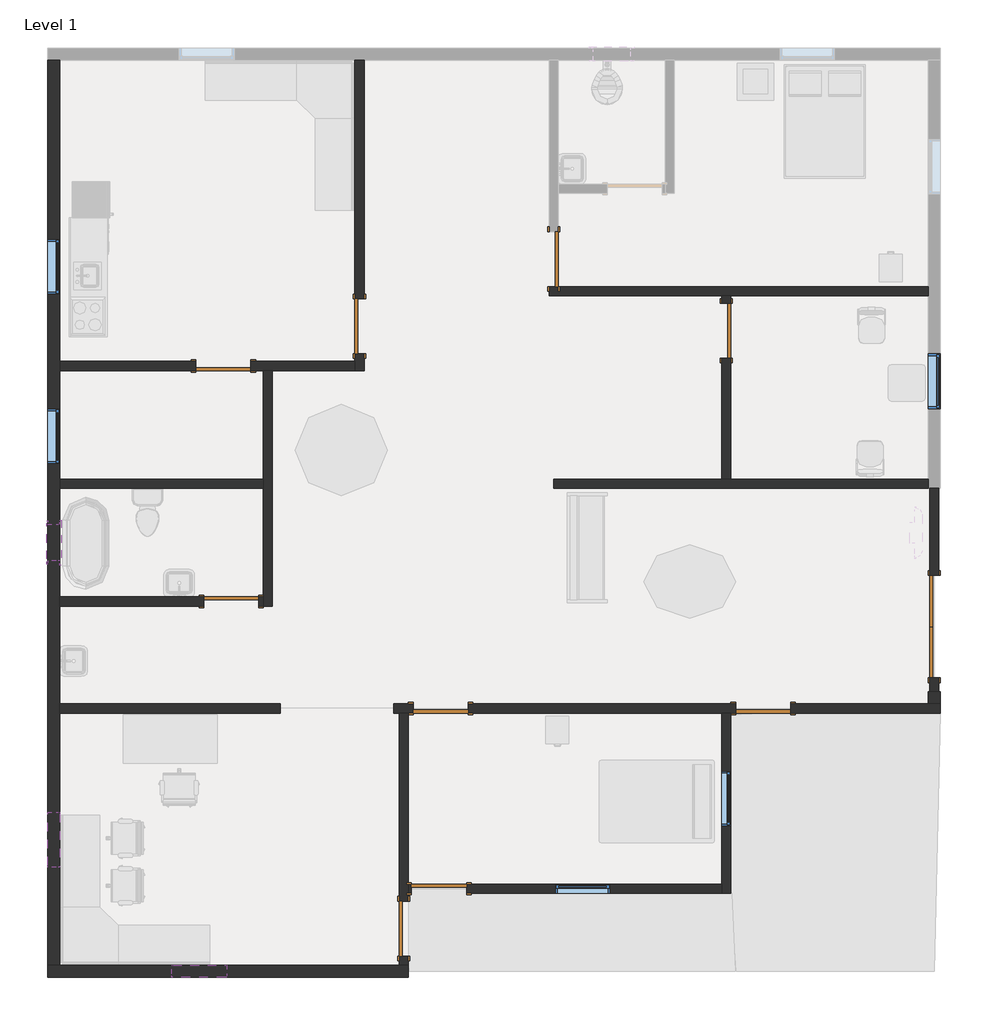
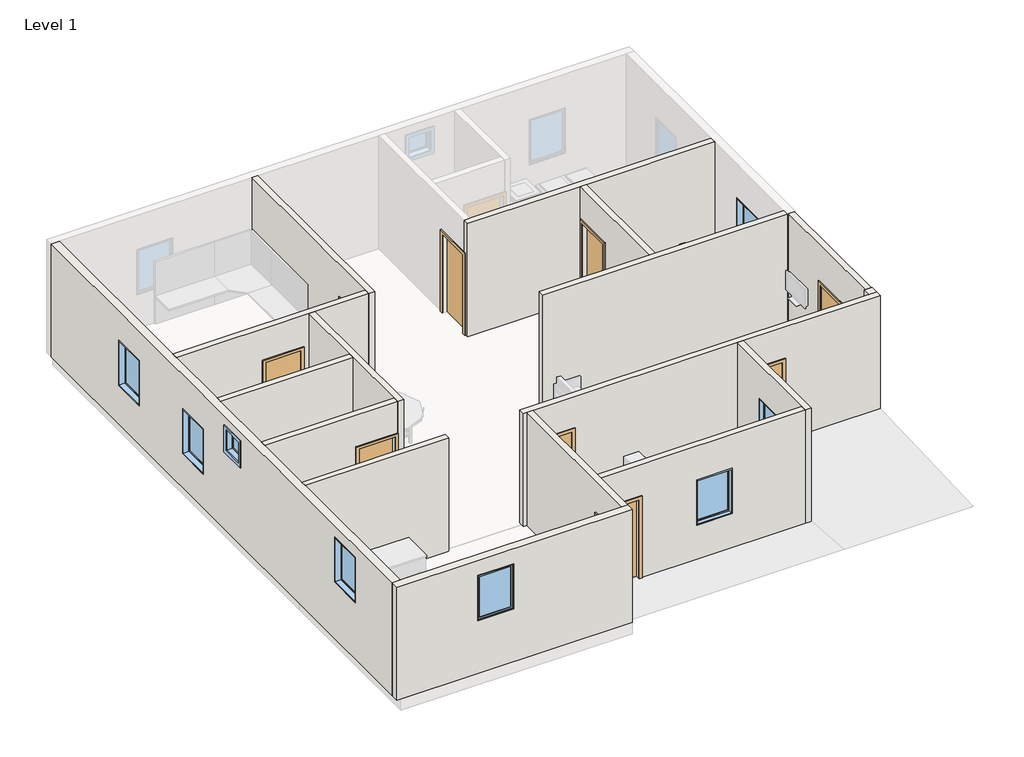
# One storey, part 1 of 2: 17 walls, 10 doors, 8 windows.
"""IFC4 building model written with IfcOpenShell, lengths in millimetres."""

from ifc_helpers import new_model, si_unit, frame, origin, origin_with_axes, place, context, project, spatial, polyline, outline, extrude, faceted_brep, transform, mapped, element, save
from components import m_door_double_flush_panel_1700_x_2000mm_b668bbd0, door_686f89d2, door_16372e1c, window_e2841890, window_d657a5cb, window_e41d21a6

model = new_model("IFC4")

# Units and contexts
model_context = context("Model", 3, world=origin())
ifc_project = project(units=[si_unit("LENGTHUNIT", "METRE", prefix="MILLI")], contexts=[model_context])

# Site, building, storey
site = spatial("IfcSite", under=ifc_project)
building = spatial("IfcBuilding", under=site)
storey = spatial("IfcBuildingStorey", under=building, Name="Level 1", Elevation=0.0)

# Doors
placement = place(None, origin())
m_door_double_flush_panel_1700_x_2000mm_shape = m_door_double_flush_panel_1700_x_2000mm_b668bbd0(model_context)
element("IfcDoor", 1, ObjectType="M_Door-Double-Flush_Panel : 1700 x 2000mm", at=placement, inside=storey, context=model_context, shape_type="MappedRepresentation", body=[
    mapped(m_door_double_flush_panel_1700_x_2000mm_shape, transform((-650.2737976, 1065.150395, 0.0), x_axis=(0.0, 1.0, 0.0), y_axis=(-1.0, 0.0, 0.0), z_axis=(0.0, 0.0, 1.0))),
])
door_shape = door_686f89d2(model_context)
element("IfcDoor", 2, ObjectType="Single-Flush : 36\" x 84\"", at=placement, inside=storey, context=model_context, shape_type="MappedRepresentation", body=[
    mapped(door_shape, transform((-10200.6737976, 6056.250395, 0.0), x_axis=(0.0, -1.0, 0.0), y_axis=(1.0, 0.0, 0.0), z_axis=(0.0, 0.0, 1.0))),
])
element("IfcDoor", 3, ObjectType="Single-Flush : 36\" x 84\"", at=placement, inside=storey, context=model_context, shape_type="MappedRepresentation", body=[
    mapped(door_shape, transform((-12461.2737976, 5395.850395, 0.0), x_axis=(1.0, 0.0, 0.0), y_axis=(0.0, 1.0, 0.0), z_axis=(0.0, 0.0, 1.0))),
])
element("IfcDoor", 4, ObjectType="Single-Flush : 36\" x 84\"", at=placement, inside=storey, context=model_context, shape_type="MappedRepresentation", body=[
    mapped(door_shape, transform((-9464.0737976, -3951.349605, 0.0), x_axis=(0.0, -1.0, 0.0), y_axis=(1.0, 0.0, 0.0), z_axis=(0.0, 0.0, 1.0))),
])
element("IfcDoor", 5, ObjectType="Single-Flush : 36\" x 84\"", at=placement, inside=storey, context=model_context, shape_type="MappedRepresentation", body=[
    mapped(door_shape, transform((-8879.8737976, -3290.949605, 0.0), x_axis=(-1.0, 0.0, 0.0), y_axis=(0.0, -1.0, 0.0), z_axis=(0.0, 0.0, 1.0))),
])
element("IfcDoor", 6, ObjectType="Single-Flush : 36\" x 84\"", at=placement, inside=storey, context=model_context, shape_type="MappedRepresentation", body=[
    mapped(door_shape, transform((-4104.6737976, 5980.050395, 0.0), x_axis=(0.0, 1.0, 0.0), y_axis=(-1.0, 0.0, 0.0), z_axis=(0.0, 0.0, 1.0))),
])
door_2_shape = door_16372e1c(model_context)
element("IfcDoor", 7, ObjectType="Single-Flush : 36\" x 84\"", at=placement, inside=storey, context=model_context, shape_type="MappedRepresentation", body=[
    mapped(door_2_shape, transform((-12334.2737976, 1484.250395, 0.0), x_axis=(1.0, 0.0, 0.0), y_axis=(0.0, 1.0, 0.0), z_axis=(0.0, 0.0, 1.0))),
])
element("IfcDoor", 8, ObjectType="Single-Flush : 36\" x 84\"", at=placement, inside=storey, context=model_context, shape_type="MappedRepresentation", body=[
    mapped(door_2_shape, transform((-8854.4737976, -293.749605, 0.0), x_axis=(-1.0, 0.0, 0.0), y_axis=(0.0, -1.0, 0.0), z_axis=(0.0, 0.0, 1.0))),
])
element("IfcDoor", 9, ObjectType="Single-Flush : 36\" x 84\"", at=placement, inside=storey, context=model_context, shape_type="MappedRepresentation", body=[
    mapped(door_2_shape, transform((-3495.0737976, -293.749605, 0.0), x_axis=(-1.0, 0.0, 0.0), y_axis=(0.0, -1.0, 0.0), z_axis=(0.0, 0.0, 1.0))),
])
element("IfcDoor", 10, ObjectType="Single-Flush : 36\" x 84\"", at=placement, inside=storey, context=model_context, shape_type="MappedRepresentation", body=[
    mapped(door_2_shape, transform((-6974.8737976, 7173.850395, 0.0), x_axis=(0.0, -1.0, 0.0), y_axis=(1.0, 0.0, 0.0), z_axis=(0.0, 0.0, 1.0))),
])

# Walls
element("IfcWall", 11, ObjectType="Generic - 8\"", at=placement, inside=storey, context=model_context, shape_type="Brep", body=[
    faceted_brep([(-15179.0737976, -4560.949605, 0.0), (-15179.0737976, -369.949605, 0.0), (-15179.0737976, -217.549605, 0.0), (-15179.0737976, 1408.050395, 0.0), (-15179.0737976, 1560.450395, 0.0), (-15179.0737976, 3363.850395, 0.0), (-15179.0737976, 3516.250395, 0.0), (-15179.0737976, 5319.650395, 0.0), (-15179.0737976, 5472.050395, 0.0), (-15179.0737976, 10475.850395, 0.0), (-15179.0737976, 10475.850395, 3048.0), (-15179.0737976, 5472.050395, 3048.0), (-15179.0737976, 5319.650395, 3048.0), (-15179.0737976, 3516.250395, 3048.0), (-15179.0737976, 3363.850395, 3048.0), (-15179.0737976, 1560.450395, 3048.0), (-15179.0737976, 1408.050395, 3048.0), (-15179.0737976, -217.549605, 3048.0), (-15179.0737976, -369.949605, 3048.0), (-15179.0737976, -4560.949605, 3048.0), (-15179.0737976, 6589.650395, 2260.6), (-15179.0737976, 7504.050395, 2260.6), (-15179.0737976, 7504.050395, 1041.4), (-15179.0737976, 6589.650395, 1041.4), (-15179.0737976, 3770.250395, 2133.6), (-15179.0737976, 4684.650395, 2133.6), (-15179.0737976, 4684.650395, 914.4), (-15179.0737976, 3770.250395, 914.4), (-15179.0737976, -2935.349605, 2743.2), (-15179.0737976, -2020.949605, 2743.2), (-15179.0737976, -2020.949605, 1524.0), (-15179.0737976, -2935.349605, 1524.0), (-15179.0737976, 2157.350395, 2768.6), (-15179.0737976, 2766.950395, 2768.6), (-15179.0737976, 2766.950395, 2159.0), (-15179.0737976, 2157.350395, 2159.0), (-15382.2737976, -4560.949605, 0.0), (-15382.2737976, -4560.949605, 3048.0), (-15382.2737976, 10475.850395, 3048.0), (-15382.2737976, 10475.850395, 0.0), (-15382.2737976, 6589.650395, 2260.6), (-15382.2737976, 6589.650395, 1041.4), (-15382.2737976, 7504.050395, 1041.4), (-15382.2737976, 7504.050395, 2260.6), (-15382.2737976, 3770.250395, 2133.6), (-15382.2737976, 3770.250395, 914.4), (-15382.2737976, 4684.650395, 914.4), (-15382.2737976, 4684.650395, 2133.6), (-15382.2737976, -2935.349605, 2743.2), (-15382.2737976, -2935.349605, 1524.0), (-15382.2737976, -2020.949605, 1524.0), (-15382.2737976, -2020.949605, 2743.2), (-15382.2737976, 2157.350395, 2768.6), (-15382.2737976, 2157.350395, 2159.0), (-15382.2737976, 2766.950395, 2159.0), (-15382.2737976, 2766.950395, 2768.6)], [[[0, 1, 2, 3, 4, 5, 6, 7, 8, 9, 10, 11, 12, 13, 14, 15, 16, 17, 18, 19], [20, 21, 22, 23], [24, 25, 26, 27], [28, 29, 30, 31], [32, 33, 34, 35]], [[36, 37, 38, 39], [40, 41, 42, 43], [44, 45, 46, 47], [48, 49, 50, 51], [52, 53, 54, 55]], [[9, 8, 7, 6, 5, 4, 3, 2, 1, 0, 36, 39]], [[19, 18, 17, 16, 15, 14, 13, 12, 11, 10, 38, 37]], [[10, 9, 39, 38]], [[0, 19, 37, 36]], [[41, 40, 20, 23]], [[42, 41, 23, 22]], [[43, 42, 22, 21]], [[40, 43, 21, 20]], [[45, 44, 24, 27]], [[46, 45, 27, 26]], [[47, 46, 26, 25]], [[44, 47, 25, 24]], [[49, 48, 28, 31]], [[50, 49, 31, 30]], [[51, 50, 30, 29]], [[48, 51, 29, 28]], [[53, 52, 32, 35]], [[54, 53, 35, 34]], [[55, 54, 34, 33]], [[52, 55, 33, 32]]]),
])
element("IfcWall", 12, ObjectType="Generic - 8\"", at=placement, inside=storey, context=model_context, shape_type="Brep", body=[
    faceted_brep([(-9387.8737976, -4560.949605, 0.0), (-9540.2737976, -4560.949605, 0.0), (-15179.0737976, -4560.949605, 0.0), (-15382.2737976, -4560.949605, 0.0), (-15382.2737976, -4560.949605, 3048.0), (-15179.0737976, -4560.949605, 3048.0), (-9540.2737976, -4560.949605, 3048.0), (-9387.8737976, -4560.949605, 3048.0), (-13324.8737976, -4560.949605, 2641.6), (-13324.8737976, -4560.949605, 1422.4), (-12410.4737976, -4560.949605, 1422.4), (-12410.4737976, -4560.949605, 2641.6), (-9387.8737976, -4764.149605, 0.0), (-9387.8737976, -4764.149605, 3048.0), (-15382.2737976, -4764.149605, 3048.0), (-15382.2737976, -4764.149605, 0.0), (-13324.8737976, -4764.149605, 2641.6), (-12410.4737976, -4764.149605, 2641.6), (-12410.4737976, -4764.149605, 1422.4), (-13324.8737976, -4764.149605, 1422.4)], [[[0, 1, 2, 3, 4, 5, 6, 7], [8, 9, 10, 11]], [[12, 13, 14, 15], [16, 17, 18, 19]], [[3, 2, 1, 0, 12, 15]], [[7, 6, 5, 4, 14, 13]], [[4, 3, 15, 14]], [[0, 7, 13, 12]], [[9, 8, 16, 19]], [[10, 9, 19, 18]], [[11, 10, 18, 17]], [[8, 11, 17, 16]]]),
])
element("IfcWall", 13, ObjectType="Generic - 8\"", at=placement, inside=storey, context=model_context, shape_type="Brep", body=[
    faceted_brep([(-751.8737976, -14.349605, 0.0), (-751.8737976, -217.549605, 0.0), (-751.8737976, -217.549605, 3048.0), (-751.8737976, -14.349605, 3048.0), (-548.6737976, -14.349605, 0.0), (-548.6737976, -14.349605, 3048.0), (-548.6737976, -217.549605, 3048.0), (-548.6737976, -217.549605, 0.0), (-726.4737976, -14.349605, 0.0), (-574.0737976, -14.349605, 0.0), (-574.0737976, -14.349605, 3048.0), (-726.4737976, -14.349605, 3048.0)], [[[0, 1, 2, 3]], [[4, 5, 6, 7]], [[1, 0, 8, 9, 4, 7]], [[3, 2, 6, 5, 10, 11]], [[0, 3, 11, 10, 5, 4, 9, 8]], [[2, 1, 7, 6]]]),
])
element("IfcWall", 14, ObjectType="INNER WALL 6\"", at=placement, inside=storey, context=model_context, shape_type="Brep", body=[
    faceted_brep([(-10276.8737976, 5599.050395, 2133.6), (-10276.8737976, 5599.050395, 0.0), (-10276.8737976, 5472.050395, 0.0), (-10276.8737976, 5319.650395, 0.0), (-10276.8737976, 5319.650395, 3048.0), (-10276.8737976, 5472.050395, 3048.0), (-10276.8737976, 10475.850395, 3048.0), (-10276.8737976, 10475.850395, 0.0), (-10276.8737976, 6513.450395, 0.0), (-10276.8737976, 6513.450395, 2133.6), (-10124.4737976, 5319.650395, 0.0), (-10124.4737976, 5599.050395, 0.0), (-10124.4737976, 5599.050395, 2133.6), (-10124.4737976, 6513.450395, 2133.6), (-10124.4737976, 6513.450395, 0.0), (-10124.4737976, 10475.850395, 0.0), (-10124.4737976, 10475.850395, 3048.0), (-10124.4737976, 5319.650395, 3048.0)], [[[0, 1, 2, 3, 4, 5, 6, 7, 8, 9]], [[10, 11, 12, 13, 14, 15, 16, 17]], [[8, 7, 15, 14]], [[3, 2, 1, 11, 10]], [[6, 5, 4, 17, 16]], [[7, 6, 16, 15]], [[4, 3, 10, 17]], [[12, 11, 1, 0]], [[13, 12, 0, 9]], [[14, 13, 9, 8]]]),
])
element("IfcWall", 15, ObjectType="INNER WALL 6\"", at=placement, inside=storey, context=model_context, shape_type="Brep", body=[
    faceted_brep([(-10276.8737976, 5472.050395, 0.0), (-12004.0737976, 5472.050395, 0.0), (-12004.0737976, 5472.050395, 2133.6), (-12918.4737976, 5472.050395, 2133.6), (-12918.4737976, 5472.050395, 0.0), (-15179.0737976, 5472.050395, 0.0), (-15179.0737976, 5472.050395, 3048.0), (-10276.8737976, 5472.050395, 3048.0), (-12004.0737976, 5319.650395, 2133.6), (-12004.0737976, 5319.650395, 0.0), (-11800.8737976, 5319.650395, 0.0), (-11648.4737976, 5319.650395, 0.0), (-10276.8737976, 5319.650395, 0.0), (-10276.8737976, 5319.650395, 3048.0), (-11648.4737976, 5319.650395, 3048.0), (-11800.8737976, 5319.650395, 3048.0), (-15179.0737976, 5319.650395, 3048.0), (-15179.0737976, 5319.650395, 0.0), (-12918.4737976, 5319.650395, 0.0), (-12918.4737976, 5319.650395, 2133.6)], [[[0, 1, 2, 3, 4, 5, 6, 7]], [[8, 9, 10, 11, 12, 13, 14, 15, 16, 17, 18, 19]], [[18, 17, 5, 4]], [[12, 11, 10, 9, 1, 0]], [[7, 6, 16, 15, 14, 13]], [[0, 7, 13, 12]], [[6, 5, 17, 16]], [[2, 1, 9, 8]], [[3, 2, 8, 19]], [[4, 3, 19, 18]]]),
])
element("IfcWall", 16, ObjectType="INNER WALL 6\"", at=placement, inside=storey, context=model_context, shape_type="Brep", body=[
    faceted_brep([(-11800.8737976, 5319.650395, 0.0), (-11800.8737976, 3516.250395, 0.0), (-11800.8737976, 3363.850395, 0.0), (-11800.8737976, 1560.450395, 0.0), (-11800.8737976, 1408.050395, 0.0), (-11800.8737976, 1408.050395, 3048.0), (-11800.8737976, 1560.450395, 3048.0), (-11800.8737976, 3363.850395, 3048.0), (-11800.8737976, 3516.250395, 3048.0), (-11800.8737976, 5319.650395, 3048.0), (-11648.4737976, 5319.650395, 0.0), (-11648.4737976, 5319.650395, 3048.0), (-11648.4737976, 1408.050395, 3048.0), (-11648.4737976, 1408.050395, 0.0)], [[[0, 1, 2, 3, 4, 5, 6, 7, 8, 9]], [[10, 11, 12, 13]], [[4, 3, 2, 1, 0, 10, 13]], [[9, 8, 7, 6, 5, 12, 11]], [[0, 9, 11, 10]], [[5, 4, 13, 12]]]),
])
element("IfcWall", 17, ObjectType="INNER WALL 6\"", at=placement, inside=storey, context=model_context, shape_type="SweptSolid", body=[
    extrude(outline(polyline([(2133.6, -11877.0737976), (0.0, -11877.0737976), (0.0, -11800.8737976), (3048.0, -11800.8737976), (3048.0, -15179.0737976), (0.0, -15179.0737976), (0.0, -12791.4737976), (2133.6, -12791.4737976), (2133.6, -11877.0737976)])), frame((0.0, 1408.050395, 0.0), z_axis=(0.0, 1.0, 0.0), x_axis=(0.0, 0.0, 1.0)), (0.0, 0.0, 1.0), 152.4),
])
element("IfcWall", 18, ObjectType="INNER WALL 6\"", at=placement, inside=storey, context=model_context, shape_type="SweptSolid", body=[
    extrude(outline(polyline([(-15179.0737976, 3516.250395), (-11800.8737976, 3516.250395), (-11800.8737976, 3363.850395), (-15179.0737976, 3363.850395), (-15179.0737976, 3516.250395)])), origin_with_axes(), (0.0, 0.0, 1.0), 3048.0),
])
element("IfcWall", 19, ObjectType="INNER WALL 6\"", at=placement, inside=storey, context=model_context, shape_type="SweptSolid", body=[
    extrude(outline(polyline([(-11521.4737976, -369.949605), (-15179.0737976, -369.949605), (-15179.0737976, -217.549605), (-11521.4737976, -217.549605), (-11521.4737976, -369.949605)])), origin_with_axes(), (0.0, 0.0, 1.0), 3048.0),
])
element("IfcWall", 20, ObjectType="INNER WALL 6\"", at=placement, inside=storey, context=model_context, shape_type="Brep", body=[
    faceted_brep([(-9540.2737976, -4408.549605, 2133.6), (-9540.2737976, -4408.549605, 0.0), (-9540.2737976, -4560.949605, 0.0), (-9540.2737976, -4560.949605, 3048.0), (-9540.2737976, -369.949605, 3048.0), (-9540.2737976, -369.949605, 0.0), (-9540.2737976, -3494.149605, 0.0), (-9540.2737976, -3494.149605, 2133.6), (-9387.8737976, -4560.949605, 0.0), (-9387.8737976, -4408.549605, 0.0), (-9387.8737976, -4408.549605, 2133.6), (-9387.8737976, -3494.149605, 2133.6), (-9387.8737976, -3494.149605, 0.0), (-9387.8737976, -3367.149605, 0.0), (-9387.8737976, -3214.749605, 0.0), (-9387.8737976, -369.949605, 0.0), (-9387.8737976, -369.949605, 3048.0), (-9387.8737976, -3214.749605, 3048.0), (-9387.8737976, -3367.149605, 3048.0), (-9387.8737976, -4560.949605, 3048.0)], [[[0, 1, 2, 3, 4, 5, 6, 7]], [[8, 9, 10, 11, 12, 13, 14, 15, 16, 17, 18, 19]], [[6, 5, 15, 14, 13, 12]], [[2, 1, 9, 8]], [[4, 3, 19, 18, 17, 16]], [[5, 4, 16, 15]], [[10, 9, 1, 0]], [[11, 10, 0, 7]], [[12, 11, 7, 6]], [[3, 2, 8, 19]]]),
])
element("IfcWall", 21, ObjectType="INNER WALL 6\"", at=placement, inside=storey, context=model_context, shape_type="Brep", body=[
    faceted_brep([(-4180.8737976, -369.949605, 0.0), (-4180.8737976, -3214.749605, 0.0), (-4180.8737976, -3367.149605, 0.0), (-4180.8737976, -3367.149605, 3048.0), (-4180.8737976, -3214.749605, 3048.0), (-4180.8737976, -369.949605, 3048.0), (-4180.8737976, -2249.549605, 2133.6), (-4180.8737976, -2249.549605, 914.4), (-4180.8737976, -1335.149605, 914.4), (-4180.8737976, -1335.149605, 2133.6), (-4028.4737976, -369.949605, 0.0), (-4028.4737976, -369.949605, 3048.0), (-4028.4737976, -3367.149605, 3048.0), (-4028.4737976, -3367.149605, 0.0), (-4028.4737976, -2249.549605, 2133.6), (-4028.4737976, -1335.149605, 2133.6), (-4028.4737976, -1335.149605, 914.4), (-4028.4737976, -2249.549605, 914.4)], [[[0, 1, 2, 3, 4, 5], [6, 7, 8, 9]], [[10, 11, 12, 13], [14, 15, 16, 17]], [[2, 1, 0, 10, 13]], [[5, 4, 3, 12, 11]], [[3, 2, 13, 12]], [[0, 5, 11, 10]], [[7, 6, 14, 17]], [[8, 7, 17, 16]], [[9, 8, 16, 15]], [[6, 9, 15, 14]]]),
])
element("IfcWall", 22, ObjectType="INNER WALL 6\"", at=placement, inside=storey, context=model_context, shape_type="Brep", body=[
    faceted_brep([(-6974.8737976, 3363.850395, 0.0), (-751.8737976, 3363.850395, 0.0), (-751.8737976, 3363.850395, 3048.0), (-6974.8737976, 3363.850395, 3048.0), (-6974.8737976, 3516.250395, 0.0), (-6974.8737976, 3516.250395, 3048.0), (-4180.8737976, 3516.250395, 3048.0), (-4028.4737976, 3516.250395, 3048.0), (-751.8737976, 3516.250395, 3048.0), (-751.8737976, 3516.250395, 0.0), (-4028.4737976, 3516.250395, 0.0), (-4180.8737976, 3516.250395, 0.0)], [[[0, 1, 2, 3]], [[4, 5, 6, 7, 8, 9, 10, 11]], [[1, 0, 4, 11, 10, 9]], [[3, 2, 8, 7, 6, 5]], [[0, 3, 5, 4]], [[2, 1, 9, 8]]]),
])
element("IfcWall", 23, ObjectType="INNER WALL 6\"", at=placement, inside=storey, context=model_context, shape_type="SweptSolid", body=[
    extrude(outline(polyline([(6564.250395, 0.0), (6437.250395, 0.0), (6437.250395, 2133.6), (5522.850395, 2133.6), (5522.850395, 0.0), (3516.250395, 0.0), (3516.250395, 3048.0), (6564.250395, 3048.0), (6564.250395, 0.0)])), frame((-4180.8737976, 0.0, 0.0), z_axis=(1.0, 0.0, 0.0), x_axis=(0.0, 1.0, 0.0)), (0.0, 0.0, 1.0), 152.4),
])
element("IfcWall", 24, ObjectType="INNER WALL 6\"", at=placement, inside=storey, context=model_context, shape_type="Brep", body=[
    faceted_brep([(-7051.0737976, 6564.250395, 0.0), (-4180.8737976, 6564.250395, 0.0), (-4028.4737976, 6564.250395, 0.0), (-751.8737976, 6564.250395, 0.0), (-751.8737976, 6564.250395, 3048.0), (-4028.4737976, 6564.250395, 3048.0), (-4180.8737976, 6564.250395, 3048.0), (-7051.0737976, 6564.250395, 3048.0), (-7051.0737976, 6716.650395, 0.0), (-7051.0737976, 6716.650395, 2133.6), (-7051.0737976, 6716.650395, 3048.0), (-6898.6737976, 6716.650395, 3048.0), (-751.8737976, 6716.650395, 3048.0), (-751.8737976, 6716.650395, 0.0)], [[[0, 1, 2, 3, 4, 5, 6, 7]], [[8, 9, 10, 11, 12, 13]], [[3, 2, 1, 0, 8, 13]], [[7, 6, 5, 4, 12, 11, 10]], [[4, 3, 13, 12]], [[0, 7, 10, 9, 8]]]),
])
element("IfcWall", 25, ObjectType="INNER WALL 6\"", at=placement, inside=storey, context=model_context, shape_type="SweptSolid", body=[
    extrude(outline(polyline([(0.0, -9387.8737976), (0.0, -9337.0737976), (2133.6, -9337.0737976), (2133.6, -8422.6737976), (0.0, -8422.6737976), (0.0, -4180.8737976), (3048.0, -4180.8737976), (3048.0, -9387.8737976), (0.0, -9387.8737976)]), holes=[polyline([(2133.6, -6035.0737976), (914.4, -6035.0737976), (914.4, -6949.4737976), (2133.6, -6949.4737976), (2133.6, -6035.0737976)])]), frame((0.0, -3367.149605, 0.0), z_axis=(0.0, 1.0, 0.0), x_axis=(0.0, 0.0, 1.0)), (0.0, 0.0, 1.0), 152.4),
])
element("IfcWall", 26, ObjectType="INNER WALL 6\"", at=placement, inside=storey, context=model_context, shape_type="Brep", body=[
    faceted_brep([(-8397.2737976, -369.949605, 0.0), (-4180.8737976, -369.949605, 0.0), (-4028.4737976, -369.949605, 0.0), (-3952.2737976, -369.949605, 0.0), (-3952.2737976, -369.949605, 2133.6), (-3037.8737976, -369.949605, 2133.6), (-3037.8737976, -369.949605, 0.0), (-548.6737976, -369.949605, 0.0), (-548.6737976, -369.949605, 3048.0), (-4028.4737976, -369.949605, 3048.0), (-4180.8737976, -369.949605, 3048.0), (-9387.8737976, -369.949605, 3048.0), (-9540.2737976, -369.949605, 3048.0), (-9629.1737976, -369.949605, 3048.0), (-9629.1737976, -369.949605, 0.0), (-9540.2737976, -369.949605, 0.0), (-9387.8737976, -369.949605, 0.0), (-9311.6737976, -369.949605, 0.0), (-9311.6737976, -369.949605, 2133.6), (-8397.2737976, -369.949605, 2133.6), (-3952.2737976, -217.549605, 2133.6), (-3952.2737976, -217.549605, 0.0), (-8397.2737976, -217.549605, 0.0), (-8397.2737976, -217.549605, 2133.6), (-9311.6737976, -217.549605, 2133.6), (-9311.6737976, -217.549605, 0.0), (-9629.1737976, -217.549605, 0.0), (-9629.1737976, -217.549605, 3048.0), (-751.8737976, -217.549605, 3048.0), (-548.6737976, -217.549605, 3048.0), (-548.6737976, -217.549605, 0.0), (-751.8737976, -217.549605, 0.0), (-3037.8737976, -217.549605, 0.0), (-3037.8737976, -217.549605, 2133.6)], [[[0, 1, 2, 3, 4, 5, 6, 7, 8, 9, 10, 11, 12, 13, 14, 15, 16, 17, 18, 19]], [[20, 21, 22, 23, 24, 25, 26, 27, 28, 29, 30, 31, 32, 33]], [[26, 25, 17, 16, 15, 14]], [[22, 21, 3, 2, 1, 0]], [[32, 31, 30, 7, 6]], [[13, 12, 11, 10, 9, 8, 29, 28, 27]], [[14, 13, 27, 26]], [[8, 7, 30, 29]], [[0, 19, 23, 22]], [[19, 18, 24, 23]], [[18, 17, 25, 24]], [[6, 5, 33, 32]], [[5, 4, 20, 33]], [[4, 3, 21, 20]]]),
])
element("IfcWall", 27, ObjectType="INNER WALL 6\"", at=placement, inside=storey, context=model_context, shape_type="SweptSolid", body=[
    extrude(outline(polyline([(-14.349605, 3048.0), (3363.850395, 3048.0), (3363.850395, 0.0), (1915.150395, 0.0), (1915.150395, 2000.0), (215.150395, 2000.0), (215.150395, 0.0), (-14.349605, 0.0), (-14.349605, 3048.0)])), frame((-726.4737976, 0.0, 0.0), z_axis=(1.0, 0.0, 0.0), x_axis=(0.0, 1.0, 0.0)), (0.0, 0.0, 1.0), 152.4),
])

# Windows
window_shape = window_e2841890(model_context)
element("IfcWindow", 28, ObjectType="Fixed : 36\" x 48\"", at=placement, inside=storey, context=model_context, shape_type="MappedRepresentation", body=[
    mapped(window_shape, transform((-15280.6737976, 7008.750395, 127.0), x_axis=(0.0, -1.0, 0.0), y_axis=(1.0, 0.0, 0.0), z_axis=(0.0, 0.0, 1.0))),
])
element("IfcWindow", 29, ObjectType="Fixed : 36\" x 48\"", at=placement, inside=storey, context=model_context, shape_type="MappedRepresentation", body=[
    mapped(window_shape, transform((-15280.6737976, 4189.350395, 0.0), x_axis=(0.0, -1.0, 0.0), y_axis=(1.0, 0.0, 0.0), z_axis=(0.0, 0.0, 1.0))),
])
element("IfcWindow", 30, ObjectType="Fixed : 36\" x 48\"", at=placement, inside=storey, context=model_context, shape_type="MappedRepresentation", body=[
    mapped(window_shape, transform((-15280.6737976, -2516.249605, 609.6), x_axis=(0.0, -1.0, 0.0), y_axis=(1.0, 0.0, 0.0), z_axis=(0.0, 0.0, 1.0))),
])
element("IfcWindow", 31, ObjectType="Fixed : 36\" x 48\"", at=placement, inside=storey, context=model_context, shape_type="MappedRepresentation", body=[
    mapped(window_shape, transform((-12905.7737976, -4662.549605, 508.0), x_axis=(-1.0, 0.0, 0.0), y_axis=(0.0, -1.0, 0.0), z_axis=(0.0, 0.0, 1.0))),
])
element("IfcWindow", 32, ObjectType="Fixed : 36\" x 48\"", at=placement, inside=storey, context=model_context, shape_type="MappedRepresentation", body=[
    mapped(window_shape, transform((-650.2737976, 5103.750395, 0.0), x_axis=(0.0, -1.0, 0.0), y_axis=(1.0, 0.0, 0.0), z_axis=(0.0, 0.0, 1.0))),
])
window_2_shape = window_d657a5cb(model_context)
element("IfcWindow", 33, ObjectType="Fixed : 36\" x 48\"", at=placement, inside=storey, context=model_context, shape_type="MappedRepresentation", body=[
    mapped(window_2_shape, transform((-6454.1737976, -3290.949605, 0.0), x_axis=(1.0, 0.0, 0.0), y_axis=(0.0, 1.0, 0.0), z_axis=(0.0, 0.0, 1.0))),
])
element("IfcWindow", 34, ObjectType="Fixed : 36\" x 48\"", at=placement, inside=storey, context=model_context, shape_type="MappedRepresentation", body=[
    mapped(window_2_shape, transform((-4104.6737976, -1830.449605, 0.0), x_axis=(0.0, -1.0, 0.0), y_axis=(1.0, 0.0, 0.0), z_axis=(0.0, 0.0, 1.0))),
])
window_3_shape = window_e41d21a6(model_context)
element("IfcWindow", 35, ObjectType="Transom with Trim : 24\" x 24\"", at=placement, inside=storey, context=model_context, shape_type="MappedRepresentation", body=[
    mapped(window_3_shape, transform((-15280.6737976, 2424.050395, 0.0), x_axis=(0.0, -1.0, 0.0), y_axis=(1.0, 0.0, 0.0), z_axis=(0.0, 0.0, 1.0))),
])

save(model, "model.ifc")

# Revit data of these elements
# Type "M_Door-Double-Flush_Panel : 1700 x 2000mm"
#   Type Mark = "8"
#   Construction Type Id = "DOOR"
#   Assembly Code = "C1020"
#   Analytic Construction = "Wooden"
#   Thickness = 0' - 1.9685"
#   Thermal Resistance (R) = 2.5876 (h·ft²·°F)/BTU
#   Swing Angle [instance default] = 90.00°
#   Panel Width = 2' - 9.46457"
#   Heat Transfer Coefficient (U) = 0.3865 BTU/(h·ft²·°F)
#   Height = 6' - 6.74016"
#   Trim Projection Ext = 0' - 0.98425"
#   Trim Projection Int = 0' - 0.98425"
#   Trim Width = 0' - 3.14961"
#   Width = 5' - 6.92913"
#   Define Thermal Properties by = 1
#   Panel Material = Wood - Birch - Solid Stained Light Low Gloss
#   Trim Material = Paint - Sienna
#   Visual Light Transmittance = 0
#   Solar Heat Gain Coefficient = 0
#   Function = (empty or 0)
#   Wall Closure = (empty or 0)
# Type "Single-Flush : 36\" x 84\""
#   Type Mark = "1"
#   Construction Type Id = "MDOOR"
#   Assembly Code = "C1020"
#   Analytic Construction = "Metal"
#   Thickness = 0' - 2"
#   Heat Transfer Coefficient (U) = 0.651978 BTU/(h·ft²·°F)
#   Height = 7' - 0"
#   Trim Projection Ext = 0' - 1"
#   Trim Projection Int = 0' - 1"
#   Trim Width = 0' - 3"
#   Width = 3' - 0"
#   Define Thermal Properties by = 1
#   Door Material = Door - Panel
#   Frame Material = Door - Frame
#   Visual Light Transmittance = 0
#   Solar Heat Gain Coefficient = 0
#   Function = (empty or 0)
#   Wall Closure = (empty or 0)
# Type "Generic - 8\""
#   Assembly Code = "B2010"
#   Layers, outside or top first: 0' - 8" no material (function 1)
# Type "INNER WALL 6\""
#   Assembly Code = "B2010"
#   Layers, outside or top first: 0' - 6" no material (function 1)
# Type "Fixed : 36\" x 48\""
#   Type Mark = "1"
#   Construction Type Id = "GSP4R"
#   Assembly Code = "B2020100"
#   Analytic Construction = "1/8 in Pilkington single glazing"
#   Visual Light Transmittance = 0.9
#   Solar Heat Gain Coefficient = 0.78
#   Heat Transfer Coefficient (U) = 0.6496 BTU/(h·ft²·°F)
#   Height = 4' - 0"
#   Default Sill Height = 3' - 0"
#   Width = 3' - 0"
#   Window Inset = 0' - 0 3/4"
#   Define Thermal Properties by = 1
#   Glass Pane Material = Glass
#   Sash Material = Sash
#   Wall Closure = (empty or 0)
# Type "Transom with Trim : 24\" x 24\""
#   Type Mark = "10"
#   Construction Type Id = "GSP4R"
#   Assembly Code = "B2020100"
#   Analytic Construction = "1/8 in Pilkington single glazing"
#   Visual Light Transmittance = 0.9
#   Solar Heat Gain Coefficient = 0.78
#   Heat Transfer Coefficient (U) = 0.6496 BTU/(h·ft²·°F)
#   Height = 2' - 0"
#   Default Sill Height = 7' - 1"
#   Trim Projection - Ext. = 0' - 0 1/2"
#   Trim Projection - Int. = 0' - 0 3/4"
#   Trim Width - Exterior = 0' - 3 1/2"
#   Trim Width - Interior = 0' - 3 1/2"
#   Width = 2' - 0"
#   Window Inset = 0' - 0 3/4"
#   Define Thermal Properties by = 1
#   Glass Pane Material = Glass
#   Sash Material = Sash
#   Trim Exterior Material = Trim
#   Trim Interior Material = Trim
#   Wall Closure = (empty or 0)
# Element 1 (IfcDoor, "M_Door-Double-Flush_Panel : 1700 x 2000mm")
#   Swing Angle = 90.00°
#   Phase Created = New Construction
#   Materials on its faces: "Paint - Sienna", "Wood - Birch - Solid Stained Light Low Gloss"
# Elements 2, 3, 4, 5, 6, 7, 8, 9, 10 (IfcDoor, "Single-Flush : 36\" x 84\"")
#   Phase Created = New Construction
#   Materials on its faces: "Door - Frame", "Door - Panel"
# Elements 11, 12, 13 (IfcWall, "Generic - 8\"")
#   Top Offset = 0' - 0"
#   Base Offset = 0' - 0"
#   Unconnected Height = 10' - 0"
#   wall height = 10' - 0"
#   Phase Created = New Construction
#   Base Constraint = Level 1
#   Materials on its faces: "Default Wall"
# Elements 14, 15, 16, 17, 18, 19, 20, 21, 22, 23, 24, 25, 26, 27 (IfcWall, "INNER WALL 6\"")
#   Top Offset = 0' - 0"
#   Base Offset = 0' - 0"
#   Unconnected Height = 10' - 0"
#   wall height = 10' - 0"
#   Phase Created = New Construction
#   Base Constraint = Level 1
#   Materials on its faces: "Default Wall"
# Element 28 (IfcWindow, "Fixed : 36\" x 48\"")
#   Mark = "2"
#   Phase Created = New Construction
#   Materials on its faces: "Sash", "Glass"
# Element 29 (IfcWindow, "Fixed : 36\" x 48\"")
#   Mark = "3"
#   Phase Created = New Construction
#   Materials on its faces: "Sash", "Glass"
# Element 30 (IfcWindow, "Fixed : 36\" x 48\"")
#   Mark = "5"
#   Phase Created = New Construction
#   Materials on its faces: "Sash", "Glass"
# Element 31 (IfcWindow, "Fixed : 36\" x 48\"")
#   Mark = "6"
#   Phase Created = New Construction
#   Materials on its faces: "Sash", "Glass"
# Element 32 (IfcWindow, "Fixed : 36\" x 48\"")
#   Mark = "10"
#   Phase Created = New Construction
#   Materials on its faces: "Sash", "Glass"
# Element 33 (IfcWindow, "Fixed : 36\" x 48\"")
#   Mark = "7"
#   Phase Created = New Construction
#   Materials on its faces: "Sash", "Glass"
# Element 34 (IfcWindow, "Fixed : 36\" x 48\"")
#   Mark = "8"
#   Phase Created = New Construction
#   Materials on its faces: "Sash", "Glass"
# Element 35 (IfcWindow, "Transom with Trim : 24\" x 24\"")
#   Mark = "13"
#   Phase Created = New Construction
#   Materials on its faces: "Sash", "Trim", "Glass"
# Materials
#   "Wood - Birch - Solid Stained Light Low Gloss": class "Wood", colour RGB 210 159 95, transparency 0, Cost = 0
#   "Paint - Sienna": colour RGB 118 70 51, transparency 0, Cost = 0
#   "Door - Panel": class "Wood", colour RGB 210 159 95, transparency 0
#   "Door - Frame": colour RGB 118 70 51, transparency 0
#   "Glass": class "Glass", colour RGB 0 128 192, transparency 0.75, Description = "Soda Lime Glass", Cost = 0
#   "Sash": class "Wood", colour RGB 224 178 126, transparency 0
#   "Trim": class "Wood", colour RGB 224 178 126, transparency 0
#   "Default Wall": colour RGB 128 128 128, transparency 0
# Room at (-8814.416, 8901.561) mm, phase "New Construction", upper level "Level 1", upper offset 10' - 0", lower offset 0' - 0"
#   Number = "10"
#   Name = "WASH AREA"
# Room at (-5691.492, 9434.245) mm, phase "New Construction", upper level "Level 1", upper offset 10' - 0", lower offset 0' - 0"
#   Number = "11"
# Room at (-2665.543, 8172.09) mm, phase "New Construction", upper level "Level 1", upper offset 10' - 0", lower offset 0' - 0"
#   Number = "12"
#   Name = "BED ROOM"
# Room at (-13037.673, 7334.606) mm, phase "New Construction", upper level "Level 1", upper offset 10' - 0", lower offset 0' - 0"
#   Number = "1"
#   Name = "KITCHEN ROOM"
# Room at (-13302.577, 2425.339) mm, phase "New Construction", upper level "Level 1", upper offset 10' - 0", lower offset 0' - 0"
#   Number = "3"
# Room at (-13761.26, 4334.856) mm, phase "New Construction", upper level "Level 1", upper offset 10' - 0", lower offset 0' - 0"
#   Number = "4"
#   Name = "STORE ROOM"
# Room at (-6709.353, -4091.234) mm, phase "New Construction", upper level "Level 1", upper offset 10' - 0", lower offset 0' - 0"
#   Number = "13"
#   Name = "VERANDA"
# Room at (-12195.061, -2829.079) mm, phase "New Construction", upper level "Level 1", upper offset 10' - 0", lower offset 0' - 0"
#   Number = "5"
#   Name = "DRAWING HALL"
# Room at (-3758.143, 1479.252) mm, phase "New Construction", upper level "Level 1", upper offset 10' - 0", lower offset 0' - 0"
#   Number = "8"
#   Name = "LIVING ROOM"
# Room at (-2665.543, 4469.7) mm, phase "New Construction", upper level "Level 1", upper offset 10' - 0", lower offset 0' - 0"
#   Number = "9"
# Room at (-6372.604, -1566.923) mm, phase "New Construction", upper level "Level 1", upper offset 10' - 0", lower offset 0' - 0"
#   Number = "6"
#   Name = "BED ROOM"
# Room at (-8814.687, 2691.7) mm, phase "New Construction", upper level "Level 1", upper offset 10' - 0", lower offset 0' - 0"
#   Number = "7"
#   Name = "DINING ROOM"
